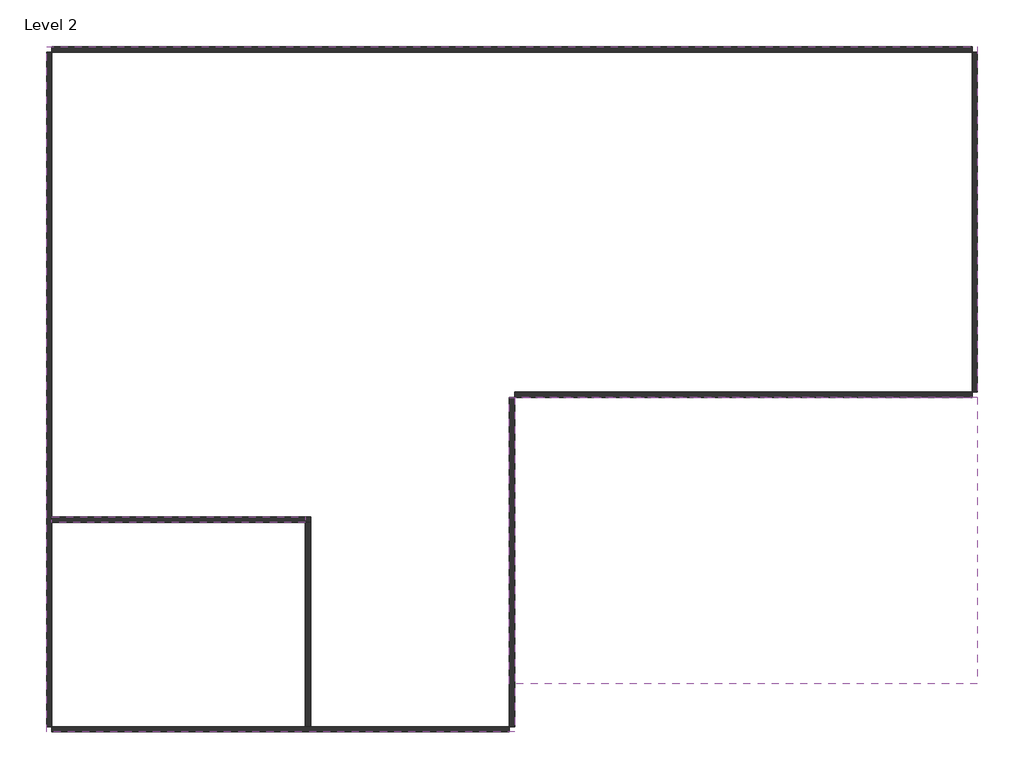
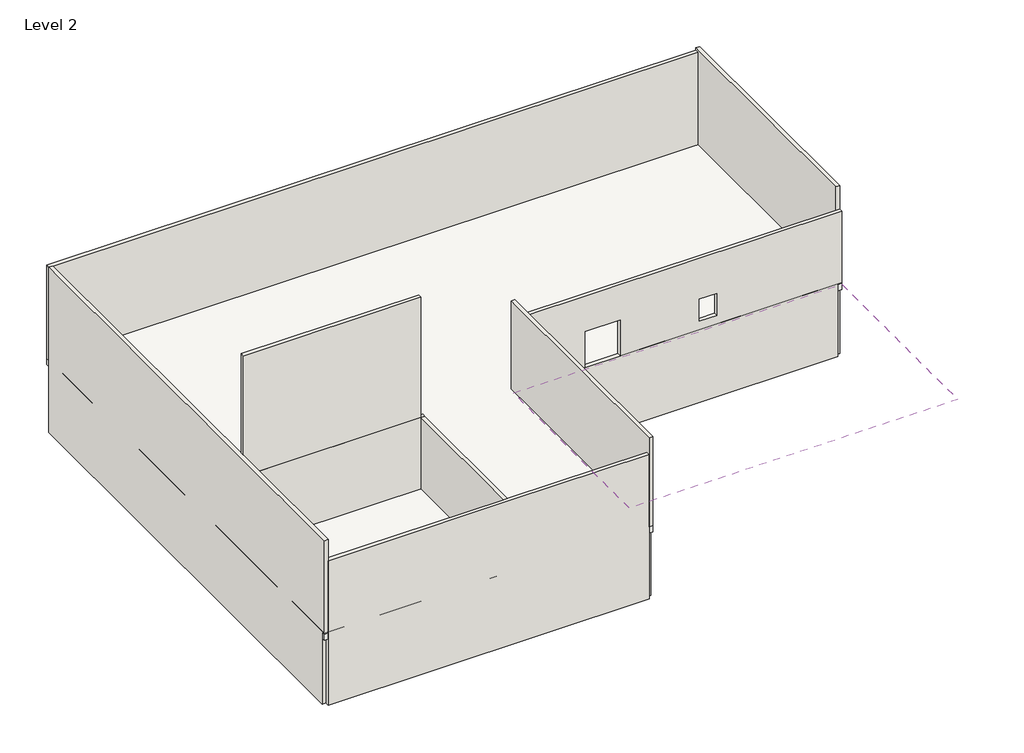
# One storey: 9 walls, 1 covering, 1 slab.
"""IFC4 building model written with IfcOpenShell, lengths in millimetres."""

from ifc_helpers import new_model, si_unit, frame, origin, place, context, project, spatial, polyline, outline, extrude, faceted_brep, element, save

model = new_model("IFC4")

# Units and contexts
model_context = context("Model", 3, world=origin())
ifc_project = project(units=[si_unit("LENGTHUNIT", "METRE", prefix="MILLI")], contexts=[model_context])

# Site, building, storey
site = spatial("IfcSite", under=ifc_project)
building = spatial("IfcBuilding", under=site)
storey = spatial("IfcBuildingStorey", under=building, Name="Level 2", Elevation=4000.0)

# Covering
placement = place(None, origin())
element("IfcCovering", 1, ObjectType="600 x 1200mm grid", at=placement, inside=storey, context=model_context, shape_type="SweptSolid", body=[
    extrude(outline(polyline([(15697.920453, 2788.3992031), (15697.920453, -7739.4271076), (-1502.079547, -7739.4271076), (-1502.079547, 2788.3992031), (15697.920453, 2788.3992031)])), frame((0.0, 0.0, 7948.0), z_axis=(0.0, 0.0, 1.0), x_axis=(1.0, 0.0, 0.0)), (0.0, 0.0, 1.0), 52.0),
])

# Slab
element("IfcSlab", 2, ObjectType="Generic Floor - 400mm", at=placement, inside=storey, context=model_context, shape_type="SweptSolid", body=[
    extrude(outline(polyline([(15697.920453, 15683.5992031), (15697.920453, 2788.3992031), (-1302.079547, 2788.3992031), (-1302.079547, -9516.4007969), (-18502.079547, -9516.4007969), (-18502.079547, 15683.5992031), (15697.920453, 15683.5992031)])), frame((0.0, 0.0, 7648.0), z_axis=(0.0, 0.0, 1.0), x_axis=(1.0, 0.0, 0.0)), (0.0, 0.0, 1.0), 400.0),
])

# Walls
element("IfcWall", 3, ObjectType="Generic - 200mm", at=placement, inside=storey, context=model_context, shape_type="Brep", body=[
    faceted_brep([(-18302.079547, 15483.5992031, 4000.0), (15497.920453, 15483.5992031, 4000.0), (15497.920453, 15483.5992031, 13159.7710807), (-18502.079547, 15483.5992031, 13159.7710807), (-18502.079547, 15483.5992031, 8000.0), (-18302.079547, 15483.5992031, 8000.0), (-18302.079547, 15683.5992031, 4000.0), (-18302.079547, 15683.5992031, 8000.0), (-18502.079547, 15683.5992031, 8000.0), (-18502.079547, 15683.5992031, 13159.7710807), (15497.920453, 15683.5992031, 13159.7710807), (15497.920453, 15683.5992031, 8000.0), (15497.920453, 15683.5992031, 4000.0)], [[[0, 1, 2, 3, 4, 5]], [[6, 7, 8, 9, 10, 11, 12]], [[1, 0, 6, 12]], [[3, 2, 10, 9]], [[4, 8, 7, 5]], [[0, 5, 7, 6]], [[4, 3, 9, 8]], [[1, 12, 11, 10, 2]]]),
])
element("IfcWall", 4, ObjectType="Generic - 200mm", at=placement, inside=storey, context=model_context, shape_type="Brep", body=[
    faceted_brep([(-18302.079547, -9316.4007969, 4000.0), (-18302.079547, -1816.4007969, 4000.0), (-18302.079547, -1616.4007969, 4000.0), (-18302.079547, 15483.5992031, 4000.0), (-18302.079547, 15483.5992031, 13172.1483612), (-18302.079547, -9516.4007969, 13172.1483612), (-18302.079547, -9516.4007969, 12000.0), (-18302.079547, -9516.4007969, 8000.0), (-18302.079547, -9316.4007969, 8000.0), (-18502.079547, -9316.4007969, 4000.0), (-18502.079547, -9316.4007969, 8000.0), (-18502.079547, -9516.4007969, 8000.0), (-18502.079547, -9516.4007969, 13172.1483612), (-18502.079547, 15483.5992031, 13172.1483612), (-18502.079547, 15483.5992031, 13159.7710807), (-18502.079547, 15483.5992031, 8000.0), (-18502.079547, 15483.5992031, 4000.0)], [[[0, 1, 2, 3, 4, 5, 6, 7, 8]], [[9, 10, 11, 12, 13, 14, 15, 16]], [[3, 2, 1, 0, 9, 16]], [[5, 4, 13, 12]], [[3, 16, 15, 14, 13, 4]], [[7, 11, 10, 8]], [[0, 8, 10, 9]], [[5, 12, 11, 7, 6]]]),
])
element("IfcWall", 5, ObjectType="Generic - 200mm", at=placement, inside=storey, context=model_context, shape_type="Brep", body=[
    faceted_brep([(-1502.079547, -9316.4007969, 12000.0), (-1502.079547, -9316.4007969, 4000.0), (-8802.079547, -9316.4007969, 4000.0), (-9002.079547, -9316.4007969, 4000.0), (-18302.079547, -9316.4007969, 4000.0), (-18302.079547, -9316.4007969, 12000.0), (-9002.079547, -9316.4007969, 12000.0), (-8802.079547, -9316.4007969, 12000.0), (-1502.079547, -9516.4007969, 4000.0), (-1502.079547, -9516.4007969, 8000.0), (-1502.079547, -9516.4007969, 12000.0), (-8802.079547, -9516.4007969, 12000.0), (-18302.079547, -9516.4007969, 12000.0), (-18302.079547, -9516.4007969, 8000.0), (-18302.079547, -9516.4007969, 4000.0)], [[[0, 1, 2, 3, 4, 5, 6, 7]], [[8, 9, 10, 11, 12, 13, 14]], [[4, 3, 2, 1, 8, 14]], [[0, 7, 6, 5, 12, 11, 10]], [[4, 14, 13, 12, 5]], [[0, 10, 9, 8, 1]]]),
])
element("IfcWall", 6, ObjectType="Generic - 200mm", at=placement, inside=storey, context=model_context, shape_type="Brep", body=[
    faceted_brep([(15497.920453, 15483.5992031, 4000.0), (15497.920453, 2988.3992031, 4000.0), (15497.920453, 2988.3992031, 13298.1092437), (15497.920453, 15683.5992031, 13298.1092437), (15497.920453, 15683.5992031, 13159.7710807), (15497.920453, 15683.5992031, 8000.0), (15497.920453, 15483.5992031, 8000.0), (15697.920453, 15483.5992031, 4000.0), (15697.920453, 15483.5992031, 8000.0), (15697.920453, 15683.5992031, 8000.0), (15697.920453, 15683.5992031, 13298.1092437), (15697.920453, 2988.3992031, 13298.1092437), (15697.920453, 2988.3992031, 12000.0), (15697.920453, 2988.3992031, 8000.0), (15697.920453, 2988.3992031, 4000.0)], [[[0, 1, 2, 3, 4, 5, 6]], [[7, 8, 9, 10, 11, 12, 13, 14]], [[1, 0, 7, 14]], [[3, 2, 11, 10]], [[5, 9, 8, 6]], [[0, 6, 8, 7]], [[5, 4, 3, 10, 9]], [[1, 14, 13, 12, 11, 2]]]),
])
element("IfcWall", 7, ObjectType="Generic - 200mm", at=placement, inside=storey, context=model_context, shape_type="Brep", body=[
    faceted_brep([(-1302.079547, -9316.4007969, 4000.0), (-1302.079547, 2788.3992031, 4000.0), (-1302.079547, 2788.3992031, 8000.0), (-1302.079547, 2988.3992031, 8000.0), (-1302.079547, 2988.3992031, 12000.0), (-1302.079547, 2988.3992031, 12922.3115167), (-1302.079547, -9516.4007969, 12922.3115167), (-1302.079547, -9516.4007969, 8000.0), (-1302.079547, -9316.4007969, 8000.0), (-1502.079547, -9316.4007969, 4000.0), (-1502.079547, -9316.4007969, 8000.0), (-1502.079547, -9516.4007969, 8000.0), (-1502.079547, -9516.4007969, 12000.0), (-1502.079547, -9516.4007969, 12922.3115167), (-1502.079547, 2988.3992031, 12922.3115167), (-1502.079547, 2988.3992031, 8000.0), (-1502.079547, 2788.3992031, 8000.0), (-1502.079547, 2788.3992031, 4000.0)], [[[0, 1, 2, 3, 4, 5, 6, 7, 8]], [[9, 10, 11, 12, 13, 14, 15, 16, 17]], [[1, 0, 9, 17]], [[6, 5, 14, 13]], [[7, 11, 10, 8]], [[0, 8, 10, 9]], [[7, 6, 13, 12, 11]], [[15, 3, 2, 16]], [[2, 1, 17, 16]], [[5, 4, 3, 15, 14]]]),
])
element("IfcWall", 8, ObjectType="Generic - 200mm", at=placement, inside=storey, context=model_context, shape_type="Brep", body=[
    faceted_brep([(-1302.079547, 2788.3992031, 4000.0), (15497.920453, 2788.3992031, 4000.0), (15497.920453, 2788.3992031, 8000.0), (15697.920453, 2788.3992031, 8000.0), (15697.920453, 2788.3992031, 12000.0), (-1302.079547, 2788.3992031, 12000.0), (2263.520453, 2788.3992031, 8048.0), (2263.520453, 2788.3992031, 10029.2), (4092.320453, 2788.3992031, 10029.2), (4092.320453, 2788.3992031, 8048.0), (8240.720453, 2788.3992031, 8514.4), (8240.720453, 2788.3992031, 9733.6), (9155.120453, 2788.3992031, 9733.6), (9155.120453, 2788.3992031, 8514.4), (15497.920453, 2988.3992031, 4000.0), (-1302.079547, 2988.3992031, 4000.0), (-1302.079547, 2988.3992031, 8000.0), (-1302.079547, 2988.3992031, 12000.0), (15697.920453, 2988.3992031, 12000.0), (15697.920453, 2988.3992031, 8000.0), (15497.920453, 2988.3992031, 8000.0), (2263.520453, 2988.3992031, 10029.2), (2263.520453, 2988.3992031, 8048.0), (4092.320453, 2988.3992031, 8048.0), (4092.320453, 2988.3992031, 10029.2), (8240.720453, 2988.3992031, 9733.6), (8240.720453, 2988.3992031, 8514.4), (9155.120453, 2988.3992031, 8514.4), (9155.120453, 2988.3992031, 9733.6)], [[[0, 1, 2, 3, 4, 5], [6, 7, 8, 9], [10, 11, 12, 13]], [[14, 15, 16, 17, 18, 19, 20], [21, 22, 23, 24], [25, 26, 27, 28]], [[1, 0, 15, 14]], [[5, 4, 18, 17]], [[3, 2, 20, 19]], [[2, 1, 14, 20]], [[4, 3, 19, 18]], [[15, 0, 5, 17, 16]], [[6, 22, 21, 7]], [[8, 24, 23, 9]], [[22, 6, 9, 23]], [[24, 8, 7, 21]], [[26, 25, 11, 10]], [[27, 26, 10, 13]], [[28, 27, 13, 12]], [[25, 28, 12, 11]]]),
])
element("IfcWall", 9, ObjectType="Generic - 200mm", at=placement, inside=storey, context=model_context, shape_type="Brep", body=[
    faceted_brep([(-8802.079547, -1616.4007969, 4000.0), (-18302.079547, -1616.4007969, 4000.0), (-18302.079547, -1616.4007969, 12000.0), (-8802.079547, -1616.4007969, 12000.0), (-8802.079547, -1816.4007969, 4000.0), (-8802.079547, -1816.4007969, 12000.0), (-9002.079547, -1816.4007969, 12000.0), (-18302.079547, -1816.4007969, 12000.0), (-18302.079547, -1816.4007969, 4000.0), (-9002.079547, -1816.4007969, 4000.0)], [[[0, 1, 2, 3]], [[4, 5, 6, 7, 8, 9]], [[1, 0, 4, 9, 8]], [[3, 2, 7, 6, 5]], [[0, 3, 5, 4]], [[1, 8, 7, 2]]]),
])
element("IfcWall", 10, ObjectType="Generic - 200mm", at=placement, inside=storey, context=model_context, shape_type="SweptSolid", body=[
    extrude(outline(polyline([(-8802.079547, -1816.4007969), (-8802.079547, -9316.4007969), (-9002.079547, -9316.4007969), (-9002.079547, -1816.4007969), (-8802.079547, -1816.4007969)])), frame((0.0, 0.0, 4000.0), z_axis=(0.0, 0.0, 1.0), x_axis=(1.0, 0.0, 0.0)), (0.0, 0.0, 1.0), 8000.0),
])
element("IfcWall", 11, ObjectType="Generic - 200mm", at=placement, inside=storey, context=model_context, shape_type="Brep", body=[
    faceted_brep([(-18302.079547, -1816.4007969, 12000.0), (-9002.079547, -1816.4007969, 12000.0), (-9002.079547, -1816.4007969, 18676.6324244), (-18302.079547, -1816.4007969, 18676.6324244), (-18302.079547, -1616.4007969, 12000.0), (-18302.079547, -1616.4007969, 18676.6324244), (-9002.079547, -1616.4007969, 18676.6324244), (-9002.079547, -1616.4007969, 18600.0), (-9002.079547, -1616.4007969, 12096.0), (-9002.079547, -1616.4007969, 12000.0)], [[[0, 1, 2, 3]], [[4, 5, 6, 7, 8, 9]], [[1, 0, 4, 9]], [[3, 2, 6, 5]], [[0, 3, 5, 4]], [[2, 1, 9, 8, 7, 6]]]),
])

save(model, "model.ifc")

# Revit data of these elements
# Type "600 x 1200mm grid"
#   built-in parameter 1002203 = 1 (stored number, unit not read)
#   built-in parameter 1002202 = 1 (stored number, unit not read)
#   Layers, outside or top first: 0' - 1.41732" "Default" (function 1); 0' - 0.62992" "Ceiling Tile 600 x 1200" (function 5)
# Type "Generic Floor - 400mm"
#   Function = 0
#   Layers, outside or top first: 1' - 3.74803" no material (function 1)
# Type "Generic - 200mm"
#   Layers, outside or top first: 0' - 7.87402" no material (function 1)
# Element 1 (IfcCovering, "600 x 1200mm grid")
#   Height Offset From Level = 12' - 11.43307"
#   Phase Created = New Construction
#   Materials on its faces: "Ceiling Tile 600 x 1200", "Default"
# Element 2 (IfcSlab, "Generic Floor - 400mm")
#   Height Offset From Level = 13' - 3.37008"
#   Phase Created = New Construction
#   Materials on its faces: "Default Roof"
# Element 3 (IfcWall, "Generic - 200mm")
#   Top Offset = 0' - 0"
#   Base Offset = 0' - 0"
#   Unconnected Height = 30' - 0.62091"
#   wall height = 30' - 0.62091"
#   Phase Created = New Construction
#   Base Constraint = Level 2
#   Materials on its faces: "Default Wall"
# Element 4 (IfcWall, "Generic - 200mm")
#   Top Offset = 0' - 0"
#   Base Offset = 0' - 0"
#   Unconnected Height = 30' - 1.1082"
#   wall height = 30' - 1.1082"
#   Phase Created = New Construction
#   Base Constraint = Level 2
#   Materials on its faces: "Default Wall"
# Elements 5, 8, 9, 10 (IfcWall, "Generic - 200mm")
#   Top Offset = 0' - 0"
#   Base Offset = 0' - 0"
#   Unconnected Height = 26' - 2.96063"
#   wall height = 26' - 2.96063"
#   Phase Created = New Construction
#   Base Constraint = Level 2
#   Materials on its faces: "Default Wall"
# Element 6 (IfcWall, "Generic - 200mm")
#   Top Offset = 0' - 0"
#   Base Offset = 0' - 0"
#   Unconnected Height = 30' - 6.06729"
#   wall height = 30' - 6.06729"
#   Phase Created = New Construction
#   Base Constraint = Level 2
#   Materials on its faces: "Default Wall"
# Element 7 (IfcWall, "Generic - 200mm")
#   Top Offset = 0' - 0"
#   Base Offset = 0' - 0"
#   Unconnected Height = 29' - 3.27211"
#   wall height = 29' - 3.27211"
#   Phase Created = New Construction
#   Base Constraint = Level 2
#   Materials on its faces: "Default Wall"
# Element 11 (IfcWall, "Generic - 200mm")
#   built-in parameter 1001111 = 26' - 2.96063"
#   Top Offset = 0' - 0"
#   Base Offset = 26' - 2.96063"
#   Unconnected Height = 21' - 10.85954"
#   wall height = 21' - 10.85954"
#   Phase Created = New Construction
#   Base Constraint = Level 2
#   Materials on its faces: "Default Wall"
# Materials
#   "Default": colour RGB 80 80 80, transparency 0
#   "Ceiling Tile 600 x 1200": class "Generic", colour RGB 179 178 175, transparency 0, Description = "Acoustic ceiling tile", Cost = 0
#   "Default Roof": colour RGB 80 80 80, transparency 0
#   "Default Wall": colour RGB 80 80 80, transparency 0
